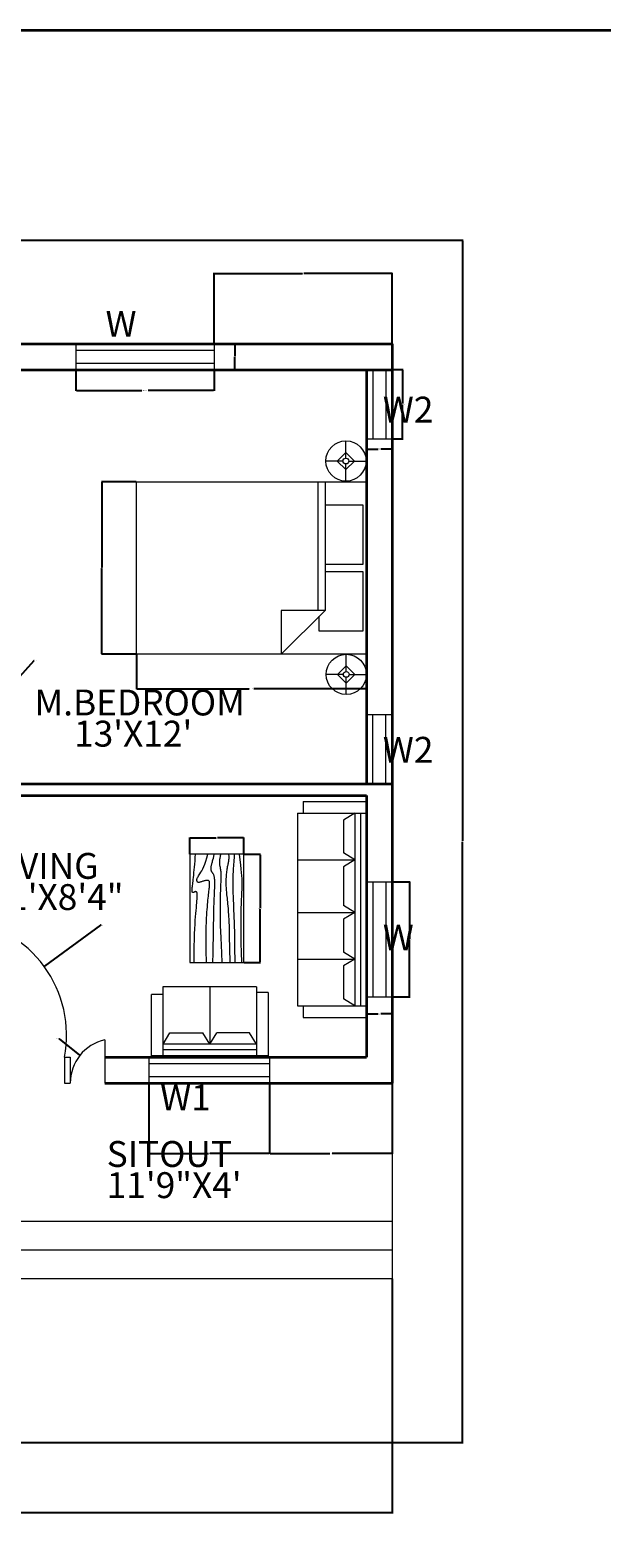
# Model space of a CAD drawing. Units: inches. Extents: x 2473 to 3664, y 1231 to 2079.
# Tile 6 of 8: x 2870 to 3069, y 1555 to 2079. Entities that reach past the tile are written whole.
import ezdxf

# ---------------------------------------------------------------- set-up
doc = ezdxf.new("R2010")
doc.units = ezdxf.units.IN
doc.linetypes.add('ACAD_ISO02W100', pattern=[15, 12, -3])
doc.layers.get('Defpoints').update_dxf_attribs({"linetype": 'ACAD_ISO02W100'})
for name, color, linetype, lineweight in [('A-ANNO-DIMS', 2, 'Continuous', 18), ('A-ANNO-IDEN', 7, 'Continuous', 18), ('A-ANNO-TTLB', 7, 'Continuous', 35), ('A-AREA-IDEN', 7, 'Continuous', 18), ('A-DOOR', 4, 'Continuous', 18), ('A-FLOR-STRS', 7, 'Continuous', 18), ('A-FURN', 8, 'Continuous', 13), ('A-GLAZ', 3, 'Continuous', 18), ('A-WALL', 7, 'Continuous', 35)]:
    doc.layers.add(name, color=color, linetype=linetype, lineweight=lineweight)
doc.styles.get("Standard").update_dxf_attribs({"font": 'arial.ttf'})
doc.dimstyles.get("Standard").update_dxf_attribs({"dimtxt": 0.18, "dimasz": 0.18, "dimexe": 0.18, "dimexo": 0.0625, "dimgap": 0.09, "dimtad": 0, "dimtih": 1, "dimtoh": 1, "dimdec": 4, "dimzin": 0, "dimdsep": 46, "dimtxsty": 'Standard', "dimcen": 0.09, "dimadec": 0, "dimazin": 0, "dimtfac": 1, "dimtdec": 4, "dimtofl": 0, "dimtmove": 0, "dimatfit": 3, "dimfxl": 1, "dimtolj": 1, "dimtzin": 0, "dimarcsym": 0})

# ---------------------------------------------------------------- blocks, each defined once
blk = doc.blocks.new('Bed - Queen')
for p, q in [((0, -80.00003), (0, 0)), ((0, 0), (59.99999, 0)), ((59.99999, 0), (59.99999, -80.00003)), ((7.99999, -1.2), (28.79998, -1.2)), ((7.99999, -14.4), (7.99999, -1.2)), ((28.79998, -1.2), (28.79998, -14.4)), ((31.19999, -1.2), (51.99999, -1.2)), ((31.19999, -14.4), (31.19999, -1.2)), ((51.99999, -1.2), (51.99999, -16.4)), ((0, -14.4), (44.8, -14.4)), ((59.99999, -29.6), (44.8, -14.4)), ((44.8, -14.4), (44.8, -29.6)), ((44.8, -16.8), (0, -16.8)), ((51.99999, -16.4), (46.79936, -16.4)), ((44.8, -29.6), (59.99999, -29.6)), ((59.99999, -80.00003), (0, -80.00003))]:
    blk.add_line(p, q)
blk = doc.blocks.new('Lamp - Table')
for p, q in [((0, 7), (0, 1)), ((-1, 0), (-7, 0)), ((0, 3), (-3, 0)), ((-3, 0), (0, -3)), ((3, 0), (0, 3)), ((0, -3), (3, 0)), ((1, 0), (7, 0)), ((0, -1), (0, -7))]:
    blk.add_line(p, q)
for radius in [7, 1]:
    blk.add_circle((0, 0), radius)
blk = doc.blocks.new('Table - Rectangular Woodgrain 60 x 30 in.')
for p, q in [((0, 0), (0, -30)), ((60, 0), (0, 0)), ((60, -30), (60, 0)), ((0, -30), (60, -30))]:
    blk.add_line(p, q)
for points in [[(0, -2.4), (4.8155, -2.418), (9.0302, -2.4688), (12.709, -2.5477), (15.9167, -2.65), (18.7181, -2.7711), (21.1781, -2.9063), (23.3616, -3.0508), (25.3333, -3.2), (27.1477, -3.3495), (28.8172, -3.4958), (30.3437, -3.636), (31.7291, -3.7667), (32.9756, -3.8849), (34.0849, -3.9875), (35.059, -4.0714), (35.9, -4.1334), (36.6114, -4.1711), (37.2041, -4.1854), (37.6906, -4.1779), (38.0833, -4.15), (38.3948, -4.1034), (38.6375, -4.0396), (38.8239, -3.9602), (38.9666, -3.8667), (39.0764, -3.7608), (39.1573, -3.6448), (39.2116, -3.521), (39.2416, -3.3917), (39.2498, -3.2593), (39.2385, -3.1261), (39.21, -2.9944), (39.1666, -2.8667), (39.111, -2.7447), (39.0468, -2.6281), (38.978, -2.5163), (38.9083, -2.4083), (38.8418, -2.3035), (38.7823, -2.201), (38.7337, -2.1001), (38.7, -2), (38.6844, -1.9003), (38.6875, -1.8021), (38.7094, -1.707), (38.75, -1.6167), (38.8094, -1.5326), (38.8875, -1.4563), (38.9844, -1.3893), (39.1, -1.3333), (39.2351, -1.2896), (39.3937, -1.2583), (39.5804, -1.2396), (39.8, -1.2333), (40.057, -1.2396), (40.3562, -1.2583), (40.7023, -1.2896), (41.1, -1.3333), (41.5547, -1.3895), (42.0755, -1.4573), (42.6721, -1.5361), (43.3542, -1.625), (44.1316, -1.7233), (45.014, -1.8302), (46.0114, -1.9449), (47.1333, -2.0667), (48.3862, -2.1947), (49.7625, -2.3281), (51.2513, -2.4663), (52.8416, -2.6083), (54.5226, -2.7535), (56.2833, -2.9011), (58.1127, -3.0501), (60, -3.2)], [(0, -9.2), (6.5759, -9.0858), (11.9385, -9.0365), (16.2527, -9.0418), (19.6833, -9.0917), (22.3952, -9.1759), (24.5531, -9.2844), (26.322, -9.4069), (27.8666, -9.5333), (29.3241, -9.6553), (30.7203, -9.7719), (32.0532, -9.8837), (33.3208, -9.9917), (34.5213, -10.0965), (35.6526, -10.199), (36.7128, -10.2999), (37.7, -10.4), (38.6129, -10.4996), (39.4531, -10.5969), (40.223, -10.6895), (40.925, -10.775), (41.5613, -10.8512), (42.1344, -10.9156), (42.6465, -10.966), (43.1, -11), (43.4976, -11.0158), (43.8437, -11.0136), (44.143, -10.9942), (44.4, -10.9583), (44.6195, -10.9069), (44.8062, -10.8406), (44.9648, -10.7603), (45.1, -10.6667), (45.2155, -10.5598), (45.3114, -10.4365), (45.3871, -10.2929), (45.4416, -10.125), (45.4743, -9.929), (45.4844, -9.7011), (45.4709, -9.4371), (45.4333, -9.1333), (45.3716, -8.7883), (45.2896, -8.4104), (45.1919, -8.0107), (45.0833, -7.6), (44.9685, -7.1893), (44.8521, -6.7896), (44.7388, -6.4117), (44.6333, -6.0667), (44.54, -5.7628), (44.4614, -5.4979), (44.4001, -5.2675), (44.3583, -5.0667), (44.3384, -4.8909), (44.3427, -4.7354), (44.3736, -4.5956), (44.4333, -4.4667), (44.5236, -4.3453), (44.6427, -4.2333), (44.7884, -4.1339), (44.9583, -4.05), (45.1501, -3.9849), (45.3614, -3.9417), (45.59, -3.9234), (45.8333, -3.9333), (46.0915, -3.9749), (46.3734, -4.0531), (46.6906, -4.1736), (47.0542, -4.3417), (47.4756, -4.5629), (47.9661, -4.8427), (48.5372, -5.1866), (49.2, -5.6), (49.9676, -6.0844), (50.8594, -6.625), (51.8965, -7.2031), (53.1, -7.8), (54.491, -8.3969), (56.0906, -8.975), (57.9199, -9.5156), (60, -10)], [(0, -12.8), (5.1847, -12.9322), (9.6213, -13.0323), (13.3963, -13.1059), (16.5958, -13.1583), (19.3063, -13.1952), (21.614, -13.2219), (23.6054, -13.2439), (25.3666, -13.2667), (26.9728, -13.2947), (28.4531, -13.3281), (29.8256, -13.3663), (31.1083, -13.4083), (32.3191, -13.4535), (33.476, -13.501), (34.597, -13.5501), (35.7, -13.6), (36.7984, -13.6497), (37.8875, -13.6979), (38.9578, -13.743), (40, -13.7833), (41.0047, -13.8174), (41.9625, -13.8438), (42.864, -13.8607), (43.7, -13.8667), (44.4631, -13.8604), (45.1552, -13.8417), (45.7801, -13.8104), (46.3416, -13.7667), (46.8439, -13.7104), (47.2906, -13.6417), (47.6858, -13.5604), (48.0333, -13.4667), (48.3375, -13.3608), (48.6042, -13.2448), (48.8396, -13.121), (49.05, -12.9917), (49.2417, -12.8593), (49.4208, -12.7261), (49.5937, -12.5944), (49.7667, -12.4667), (49.9452, -12.3451), (50.1323, -12.2313), (50.3303, -12.1268), (50.5416, -12.0333), (50.7686, -11.9524), (51.0135, -11.8854), (51.2788, -11.8341), (51.5666, -11.8), (51.8785, -11.7843), (52.2116, -11.7865), (52.562, -11.8059), (52.926, -11.8417), (53.2998, -11.8931), (53.6795, -11.9594), (54.0614, -12.0397), (54.4416, -12.1333), (54.8223, -12.2401), (55.2293, -12.3625), (55.6942, -12.5037), (56.2489, -12.6667), (56.9251, -12.8547), (57.7545, -13.0708), (58.7689, -13.3182), (60, -13.6)], [(0, -18), (5.124, -17.7273), (9.6609, -17.5057), (13.6705, -17.3303), (17.2125, -17.1958), (20.3467, -17.0973), (23.1328, -17.0297), (25.6307, -16.9878), (27.9, -16.9667), (29.9928, -16.9617), (31.9302, -16.9703), (33.7254, -16.9907), (35.3917, -17.0208), (36.9423, -17.0588), (38.3906, -17.1026), (39.7499, -17.1503), (41.0333, -17.2), (42.2519, -17.2496), (43.4073, -17.2969), (44.4986, -17.3395), (45.525, -17.375), (46.4858, -17.4012), (47.3802, -17.4156), (48.2074, -17.416), (48.9667, -17.4), (49.6583, -17.3662), (50.2872, -17.3167), (50.8595, -17.2547), (51.3812, -17.1833), (51.8584, -17.1057), (52.2971, -17.025), (52.7034, -16.9443), (53.0833, -16.8667), (53.443, -16.7951), (53.789, -16.7313), (54.128, -16.6768), (54.4666, -16.6334), (54.8115, -16.6024), (55.1693, -16.5854), (55.5465, -16.5841), (55.95, -16.6), (56.3828, -16.6337), (56.8346, -16.6823), (57.2915, -16.7418), (57.7396, -16.8084), (58.165, -16.878), (58.5539, -16.9469), (58.8924, -17.0111), (59.1666, -17.0667), (59.3679, -17.1107), (59.5078, -17.1438), (59.6032, -17.1675), (59.6708, -17.1833), (59.7275, -17.193), (59.7901, -17.1979), (59.8753, -17.1998), (60, -17.2)], [(0, -22.4), (8.0098, -22.2501), (14.4094, -22.1011), (19.4168, -21.9535), (23.25, -21.8083), (26.1269, -21.6663), (28.2656, -21.5281), (29.884, -21.3947), (31.2, -21.2667), (32.3967, -21.1448), (33.5172, -21.0292), (34.5697, -20.9198), (35.5625, -20.8167), (36.5037, -20.7198), (37.4015, -20.6292), (38.2642, -20.5448), (39.1, -20.4667), (39.9164, -20.3951), (40.7187, -20.3313), (41.5117, -20.2768), (42.3, -20.2333), (43.0883, -20.2024), (43.8812, -20.1854), (44.6836, -20.1841), (45.5, -20.2), (46.3328, -20.234), (47.1747, -20.2844), (48.0163, -20.3488), (48.8479, -20.425), (49.66, -20.5106), (50.4429, -20.6031), (51.1872, -20.7004), (51.8833, -20.8), (52.5246, -20.8999), (53.1166, -20.9995), (53.6681, -21.0983), (54.1875, -21.1958), (54.6834, -21.2919), (55.1646, -21.3859), (55.6394, -21.4777), (56.1167, -21.5667), (56.6028, -21.6515), (57.0961, -21.7266), (57.5929, -21.7852), (58.0896, -21.8208), (58.5823, -21.8268), (59.0674, -21.7964), (59.5412, -21.723), (60, -21.6)], [(0, -25.2), (8.6355, -25.0504), (15.7026, -24.9031), (21.4049, -24.7606), (25.9458, -24.625), (29.529, -24.4988), (32.3578, -24.3844), (34.6359, -24.284), (36.5667, -24.2), (38.3213, -24.1341), (39.9417, -24.0854), (41.437, -24.0523), (42.8167, -24.0333), (44.0901, -24.0268), (45.2667, -24.0313), (46.3557, -24.0451), (47.3667, -24.0667), (48.309, -24.0947), (49.1928, -24.1287), (50.0284, -24.168), (50.826, -24.2125), (51.5959, -24.2617), (52.3483, -24.3151), (53.0935, -24.3725), (53.8417, -24.4334), (54.6009, -24.497), (55.3699, -24.561), (56.1454, -24.6226), (56.9239, -24.6792), (57.7021, -24.7279), (58.4764, -24.7662), (59.2435, -24.7911), (60, -24.8)], [(0, -28.8), (5.6867, -28.6681), (10.45, -28.5698), (14.407, -28.5012), (17.675, -28.4584), (20.3711, -28.4374), (22.6125, -28.4344), (24.5164, -28.4455), (26.2, -28.4667), (27.762, -28.4947), (29.2276, -28.5281), (30.6033, -28.5663), (31.8958, -28.6084), (33.1118, -28.6535), (34.2578, -28.7011), (35.3405, -28.7501), (36.3666, -28.8), (37.3443, -28.8497), (38.288, -28.8974), (39.2137, -28.9412), (40.1375, -28.9792), (41.0753, -29.0093), (42.0432, -29.0297), (43.0572, -29.0384), (44.1333, -29.0333), (45.2936, -29.0114), (46.5843, -28.9641), (48.0579, -28.8816), (49.7666, -28.7542), (51.7629, -28.5721), (54.0989, -28.3255), (56.8272, -28.0048), (60, -27.6)]]:
    blk.add_lwpolyline(points)
blk = doc.blocks.new('GLAZ-PLAN-48')
for p, q in [((0, 9), (0, 0)), ((0, 6.75), (48, 6.75)), ((48, 9), (48, 0)), ((0, 2.25), (48, 2.25))]:
    blk.add_line(p, q)
blk = doc.blocks.new('GLAZ-PLAN-40')
for p, q in [((0, 40), (9, 40)), ((2.25, 40), (2.25, 0)), ((6.75, 40), (6.75, 0)), ((0, 0), (9, 0))]:
    blk.add_line(p, q)
blk = doc.blocks.new('GLAZ-PLAN-24-END')
for p, q in [((2.25, 24), (2.25, 0)), ((6.75, 24), (6.75, 0)), ((0, 0), (9, 0))]:
    blk.add_line(p, q)
blk = doc.blocks.new('STEPS-SITOUT-PLAN')
for p, q in [((151, 68), (151, 0)), ((0, 20), (151, 20)), ((0, 10), (151, 10)), ((0, 0), (151, 0))]:
    blk.add_line(p, q)
blk = doc.blocks.new('*D21')
at = {"layer": 'A-ANNO-DIMS', "color": 0, "lineweight": -2, "transparency": 16777216}
for p, q in [((2885.66, 1960.99), (2885.66, 1953.68)), ((2933.66, 1960.99), (2933.66, 1953.68)), ((2885.84, 1953.86), (2908.54, 1953.86)), ((2933.48, 1953.86), (2910.78, 1953.86))]:
    blk.add_line(p, q, dxfattribs=at)
at = {"layer": 'A-ANNO-DIMS', "color": 0, "transparency": 16777216}
for points in [[(2885.84, 1953.89), (2885.84, 1953.83), (2885.66, 1953.86)], [(2933.48, 1953.89), (2933.48, 1953.83), (2933.66, 1953.86)]]:
    blk.add_solid(points, dxfattribs=at)
at = {"layer": 'Defpoints', "color": 0, "transparency": 16777216}
for p in [(2885.66, 1961.06), (2933.66, 1961.06), (2933.66, 1953.86)]:
    blk.add_point(p, dxfattribs=at)
at = {"layer": 'A-ANNO-DIMS', "color": 0, "transparency": 16777216, "insert": (2909.66, 1953.86), "char_height": 0.18, "attachment_point": 5}
blk.add_mtext('\\A1;WINDOW 48 TYP.', dxfattribs=at)
blk = doc.blocks.new('*D22')
at = {"layer": 'A-ANNO-DIMS', "color": 0, "lineweight": -2, "transparency": 16777216}
for p, q in [((2933.72, 1970.06), (2941.04, 1970.06)), ((2940.86, 1969.88), (2940.86, 1965.74)), ((2933.72, 1961.06), (2941.04, 1961.06)), ((2940.86, 1961.24), (2940.86, 1965.37))]:
    blk.add_line(p, q, dxfattribs=at)
at = {"layer": 'A-ANNO-DIMS', "color": 0, "transparency": 16777216}
for points in [[(2940.83, 1969.88), (2940.89, 1969.88), (2940.86, 1970.06)], [(2940.83, 1961.24), (2940.89, 1961.24), (2940.86, 1961.06)]]:
    blk.add_solid(points, dxfattribs=at)
at = {"layer": 'Defpoints', "color": 0, "transparency": 16777216}
for p in [(2933.66, 1970.06), (2940.86, 1970.06), (2933.66, 1961.06)]:
    blk.add_point(p, dxfattribs=at)
at = {"layer": 'A-ANNO-DIMS', "color": 0, "transparency": 16777216, "insert": (2940.86, 1965.56), "char_height": 0.18, "attachment_point": 5}
blk.add_mtext('\\A1;9 TYP.', dxfattribs=at)
blk = doc.blocks.new('*D25')
at = {"layer": 'A-ANNO-DIMS', "color": 0, "lineweight": -2, "transparency": 16777216}
for p, q in [((2906.66, 1862.06), (2906.66, 1849.94)), ((2986.66, 1862.06), (2986.66, 1849.94)), ((2906.84, 1850.12), (2945.84, 1850.12)), ((2986.48, 1850.12), (2947.48, 1850.12))]:
    blk.add_line(p, q, dxfattribs=at)
at = {"layer": 'A-ANNO-DIMS', "color": 0, "transparency": 16777216}
for points in [[(2906.84, 1850.15), (2906.84, 1850.09), (2906.66, 1850.12)], [(2986.48, 1850.15), (2986.48, 1850.09), (2986.66, 1850.12)]]:
    blk.add_solid(points, dxfattribs=at)
at = {"layer": 'Defpoints', "color": 0, "transparency": 16777216}
for p in [(2906.66, 1862.12), (2986.66, 1862.12), (2986.66, 1850.12)]:
    blk.add_point(p, dxfattribs=at)
at = {"layer": 'A-ANNO-DIMS', "color": 0, "transparency": 16777216, "insert": (2946.66, 1850.12), "char_height": 0.18, "attachment_point": 5}
blk.add_mtext('\\A1;BED 80 TYP.', dxfattribs=at)
blk = doc.blocks.new('*D26')
at = {"layer": 'A-ANNO-DIMS', "color": 0, "lineweight": -2, "transparency": 16777216}
for p, q in [((2906.6, 1922.12), (2894.48, 1922.12)), ((2894.66, 1921.94), (2894.66, 1892.3)), ((2894.66, 1862.3), (2894.66, 1891.94)), ((2906.6, 1862.12), (2894.48, 1862.12))]:
    blk.add_line(p, q, dxfattribs=at)
at = {"layer": 'A-ANNO-DIMS', "color": 0, "transparency": 16777216}
for points in [[(2894.63, 1921.94), (2894.69, 1921.94), (2894.66, 1922.12)], [(2894.63, 1862.3), (2894.69, 1862.3), (2894.66, 1862.12)]]:
    blk.add_solid(points, dxfattribs=at)
at = {"layer": 'Defpoints', "color": 0, "transparency": 16777216}
for p in [(2906.66, 1922.12), (2894.66, 1862.12), (2906.66, 1862.12)]:
    blk.add_point(p, dxfattribs=at)
at = {"layer": 'A-ANNO-DIMS', "color": 0, "transparency": 16777216, "insert": (2894.66, 1892.12), "char_height": 0.18, "attachment_point": 5}
blk.add_mtext('\\A1;60 TYP.', dxfattribs=at)
blk = doc.blocks.new('*D27')
at = {"layer": 'A-ANNO-DIMS', "color": 0, "lineweight": -2, "transparency": 16777216}
for p, q in [((2995.72, 1783.06), (3001.84, 1783.06)), ((3001.66, 1782.88), (3001.66, 1763.24)), ((3001.66, 1743.24), (3001.66, 1762.87)), ((2995.72, 1743.06), (3001.84, 1743.06))]:
    blk.add_line(p, q, dxfattribs=at)
at = {"layer": 'A-ANNO-DIMS', "color": 0, "transparency": 16777216}
for points in [[(3001.63, 1782.88), (3001.69, 1782.88), (3001.66, 1783.06)], [(3001.63, 1743.24), (3001.69, 1743.24), (3001.66, 1743.06)]]:
    blk.add_solid(points, dxfattribs=at)
at = {"layer": 'Defpoints', "color": 0, "transparency": 16777216}
for p in [(2995.66, 1783.06), (3001.66, 1783.06), (2995.66, 1743.06)]:
    blk.add_point(p, dxfattribs=at)
at = {"layer": 'A-ANNO-DIMS', "color": 0, "transparency": 16777216, "insert": (3001.66, 1763.06), "char_height": 0.18, "attachment_point": 5}
blk.add_mtext('\\A1;WINDOW 40 TYP.', dxfattribs=at)
blk = doc.blocks.new('*D28')
at = {"layer": 'A-ANNO-DIMS', "color": 0, "lineweight": -2, "transparency": 16777216}
for p, q in [((2986.66, 1742.99), (2986.66, 1736.88)), ((2995.66, 1742.99), (2995.66, 1736.88)), ((2986.84, 1737.06), (2990.7, 1737.06)), ((2995.48, 1737.06), (2991.62, 1737.06))]:
    blk.add_line(p, q, dxfattribs=at)
at = {"layer": 'A-ANNO-DIMS', "color": 0, "transparency": 16777216}
for points in [[(2986.84, 1737.09), (2986.84, 1737.03), (2986.66, 1737.06)], [(2995.48, 1737.09), (2995.48, 1737.03), (2995.66, 1737.06)]]:
    blk.add_solid(points, dxfattribs=at)
at = {"layer": 'Defpoints', "color": 0, "transparency": 16777216}
for p in [(2986.66, 1743.06), (2995.66, 1743.06), (2995.66, 1737.06)]:
    blk.add_point(p, dxfattribs=at)
at = {"layer": 'A-ANNO-DIMS', "color": 0, "transparency": 16777216, "insert": (2991.16, 1737.06), "char_height": 0.18, "attachment_point": 5}
blk.add_mtext('\\A1;9 TYP.', dxfattribs=at)
blk = doc.blocks.new('*D33')
at = {"layer": 'A-ANNO-DIMS', "color": 0, "lineweight": -2, "transparency": 16777216}
for p, q in [((2995.72, 1961.06), (2999.44, 1961.06)), ((2999.26, 1960.88), (2999.26, 1949.24)), ((2999.26, 1937.24), (2999.26, 1948.87)), ((2995.72, 1937.06), (2999.44, 1937.06))]:
    blk.add_line(p, q, dxfattribs=at)
at = {"layer": 'A-ANNO-DIMS', "color": 0, "transparency": 16777216}
for points in [[(2999.23, 1960.88), (2999.29, 1960.88), (2999.26, 1961.06)], [(2999.23, 1937.24), (2999.29, 1937.24), (2999.26, 1937.06)]]:
    blk.add_solid(points, dxfattribs=at)
at = {"layer": 'Defpoints', "color": 0, "transparency": 16777216}
for p in [(2995.66, 1961.06), (2999.26, 1961.06), (2995.66, 1937.06)]:
    blk.add_point(p, dxfattribs=at)
at = {"layer": 'A-ANNO-DIMS', "color": 0, "transparency": 16777216, "insert": (2999.26, 1949.06), "char_height": 0.18, "attachment_point": 5}
blk.add_mtext('\\A1;WINDOW 24 TYP.', dxfattribs=at)
blk = doc.blocks.new('*D34')
at = {"layer": 'A-ANNO-DIMS', "color": 0, "lineweight": -2, "transparency": 16777216}
for p, q in [((2986.66, 1936.99), (2986.66, 1933.28)), ((2995.66, 1936.99), (2995.66, 1933.28)), ((2986.84, 1933.46), (2990.7, 1933.46)), ((2995.48, 1933.46), (2991.62, 1933.46))]:
    blk.add_line(p, q, dxfattribs=at)
at = {"layer": 'A-ANNO-DIMS', "color": 0, "transparency": 16777216}
for points in [[(2986.84, 1933.49), (2986.84, 1933.43), (2986.66, 1933.46)], [(2995.48, 1933.49), (2995.48, 1933.43), (2995.66, 1933.46)]]:
    blk.add_solid(points, dxfattribs=at)
at = {"layer": 'Defpoints', "color": 0, "transparency": 16777216}
for p in [(2986.66, 1937.06), (2995.66, 1937.06), (2995.66, 1933.46)]:
    blk.add_point(p, dxfattribs=at)
at = {"layer": 'A-ANNO-DIMS', "color": 0, "transparency": 16777216, "insert": (2991.16, 1933.46), "char_height": 0.18, "attachment_point": 5}
blk.add_mtext('\\A1;9 TYP.', dxfattribs=at)
blk = doc.blocks.new('*D47')
at = {"layer": 'A-ANNO-DIMS', "color": 0, "lineweight": -2, "transparency": 16777216}
for p, q in [((2944.12, 1792.62), (2949.88, 1792.62)), ((2949.7, 1792.44), (2949.7, 1773.98)), ((2949.7, 1755.15), (2949.7, 1773.61)), ((2944.12, 1754.97), (2949.88, 1754.97))]:
    blk.add_line(p, q, dxfattribs=at)
at = {"layer": 'A-ANNO-DIMS', "color": 0, "transparency": 16777216}
for points in [[(2949.67, 1792.44), (2949.73, 1792.44), (2949.7, 1792.62)], [(2949.67, 1755.15), (2949.73, 1755.15), (2949.7, 1754.97)]]:
    blk.add_solid(points, dxfattribs=at)
at = {"layer": 'Defpoints', "color": 0, "transparency": 16777216}
for p in [(2944.06, 1792.62), (2949.7, 1792.62), (2944.06, 1754.97)]:
    blk.add_point(p, dxfattribs=at)
at = {"layer": 'A-ANNO-DIMS', "color": 0, "transparency": 16777216, "insert": (2949.7, 1773.8), "char_height": 0.18, "attachment_point": 5}
blk.add_mtext('\\A1;TABLE 38', dxfattribs=at)
blk = doc.blocks.new('*D48')
at = {"layer": 'A-ANNO-DIMS', "color": 0, "lineweight": -2, "transparency": 16777216}
for p, q in [((2925.23, 1792.68), (2925.23, 1798.45)), ((2925.41, 1798.27), (2934.43, 1798.27)), ((2943.88, 1798.27), (2934.86, 1798.27)), ((2944.06, 1792.68), (2944.06, 1798.45))]:
    blk.add_line(p, q, dxfattribs=at)
at = {"layer": 'A-ANNO-DIMS', "color": 0, "transparency": 16777216}
for points in [[(2925.41, 1798.3), (2925.41, 1798.24), (2925.23, 1798.27)], [(2943.88, 1798.3), (2943.88, 1798.24), (2944.06, 1798.27)]]:
    blk.add_solid(points, dxfattribs=at)
at = {"layer": 'Defpoints', "color": 0, "transparency": 16777216}
for p in [(2925.23, 1798.27), (2925.23, 1792.62), (2944.06, 1792.62)]:
    blk.add_point(p, dxfattribs=at)
at = {"layer": 'A-ANNO-DIMS', "color": 0, "transparency": 16777216, "insert": (2934.64, 1798.27), "char_height": 0.18, "attachment_point": 5}
blk.add_mtext('\\A1;19', dxfattribs=at)
blk = doc.blocks.new('*D49')
at = {"layer": 'A-ANNO-DIMS', "color": 0, "lineweight": -2, "transparency": 16777216}
for p, q in [((2995.66, 1644.99), (2995.66, 1563.43)), ((2617.66, 1587.99), (2617.66, 1563.43)), ((2617.84, 1563.61), (2806.37, 1563.61)), ((2995.48, 1563.61), (2806.95, 1563.61))]:
    blk.add_line(p, q, dxfattribs=at)
at = {"layer": 'A-ANNO-DIMS', "color": 0, "transparency": 16777216}
for points in [[(2617.84, 1563.64), (2617.84, 1563.58), (2617.66, 1563.61)], [(2995.48, 1563.64), (2995.48, 1563.58), (2995.66, 1563.61)]]:
    blk.add_solid(points, dxfattribs=at)
at = {"layer": 'Defpoints', "color": 0, "transparency": 16777216}
for p in [(2995.66, 1645.06), (2617.66, 1588.06), (2995.66, 1563.61)]:
    blk.add_point(p, dxfattribs=at)
at = {"layer": 'A-ANNO-DIMS', "color": 0, "transparency": 16777216, "insert": (2806.66, 1563.61), "char_height": 0.18, "attachment_point": 5}
blk.add_mtext('\\A1;378', dxfattribs=at)
blk = doc.blocks.new('*D50')
at = {"layer": 'A-ANNO-DIMS', "color": 0, "lineweight": -2, "transparency": 16777216}
for p, q in [((2746.72, 2006.06), (3020.29, 2006.06)), ((3020.11, 2005.88), (3020.11, 1797.24)), ((3020.11, 1588.24), (3020.11, 1796.87)), ((2844.72, 1588.06), (3020.29, 1588.06))]:
    blk.add_line(p, q, dxfattribs=at)
at = {"layer": 'A-ANNO-DIMS', "color": 0, "transparency": 16777216}
for points in [[(3020.08, 2005.88), (3020.14, 2005.88), (3020.11, 2006.06)], [(3020.08, 1588.24), (3020.14, 1588.24), (3020.11, 1588.06)]]:
    blk.add_solid(points, dxfattribs=at)
at = {"layer": 'Defpoints', "color": 0, "transparency": 16777216}
for p in [(2746.66, 2006.06), (3020.11, 2006.06), (2844.66, 1588.06)]:
    blk.add_point(p, dxfattribs=at)
at = {"layer": 'A-ANNO-DIMS', "color": 0, "transparency": 16777216, "insert": (3020.11, 1797.06), "char_height": 0.18, "attachment_point": 5}
blk.add_mtext('\\A1;418', dxfattribs=at)
blk = doc.blocks.new('*D55')
at = {"layer": 'A-ANNO-DIMS', "color": 0, "lineweight": -2, "transparency": 16777216}
for p, q in [((2933.66, 1970.12), (2933.66, 1994.69)), ((2933.84, 1994.51), (2964.44, 1994.51)), ((2995.48, 1994.51), (2964.88, 1994.51)), ((2995.66, 1970.12), (2995.66, 1994.69))]:
    blk.add_line(p, q, dxfattribs=at)
at = {"layer": 'A-ANNO-DIMS', "color": 0, "transparency": 16777216}
for points in [[(2933.84, 1994.54), (2933.84, 1994.48), (2933.66, 1994.51)], [(2995.48, 1994.54), (2995.48, 1994.48), (2995.66, 1994.51)]]:
    blk.add_solid(points, dxfattribs=at)
at = {"layer": 'Defpoints', "color": 0, "transparency": 16777216}
for p in [(2995.66, 1994.51), (2933.66, 1970.06), (2995.66, 1970.06)]:
    blk.add_point(p, dxfattribs=at)
at = {"layer": 'A-ANNO-DIMS', "color": 0, "transparency": 16777216, "insert": (2964.66, 1994.51), "char_height": 0.18, "attachment_point": 5}
blk.add_mtext('\\A1;62', dxfattribs=at)
blk = doc.blocks.new('*D61')
at = {"layer": 'A-ANNO-DIMS', "color": 0, "lineweight": -2, "transparency": 16777216}
for p, q in [((2911.01, 1712.99), (2911.01, 1688.43)), ((2953.01, 1712.99), (2953.01, 1688.43)), ((2911.19, 1688.61), (2931.79, 1688.61)), ((2952.83, 1688.61), (2932.23, 1688.61))]:
    blk.add_line(p, q, dxfattribs=at)
at = {"layer": 'A-ANNO-DIMS', "color": 0, "transparency": 16777216}
for points in [[(2911.19, 1688.64), (2911.19, 1688.58), (2911.01, 1688.61)], [(2952.83, 1688.64), (2952.83, 1688.58), (2953.01, 1688.61)]]:
    blk.add_solid(points, dxfattribs=at)
at = {"layer": 'Defpoints', "color": 0, "transparency": 16777216}
for p in [(2911.01, 1713.06), (2953.01, 1713.06), (2911.01, 1688.61)]:
    blk.add_point(p, dxfattribs=at)
at = {"layer": 'A-ANNO-DIMS', "color": 0, "transparency": 16777216, "insert": (2932.01, 1688.61), "char_height": 0.18, "attachment_point": 5}
blk.add_mtext('\\A1;42', dxfattribs=at)
blk = doc.blocks.new('*D62')
at = {"layer": 'A-ANNO-DIMS', "color": 0, "lineweight": -2, "transparency": 16777216}
for p, q in [((2953.01, 1712.99), (2953.01, 1688.43)), ((2995.66, 1712.99), (2995.66, 1688.43)), ((2953.19, 1688.61), (2973.94, 1688.61)), ((2995.48, 1688.61), (2974.73, 1688.61))]:
    blk.add_line(p, q, dxfattribs=at)
at = {"layer": 'A-ANNO-DIMS', "color": 0, "transparency": 16777216}
for points in [[(2953.19, 1688.64), (2953.19, 1688.58), (2953.01, 1688.61)], [(2995.48, 1688.64), (2995.48, 1688.58), (2995.66, 1688.61)]]:
    blk.add_solid(points, dxfattribs=at)
at = {"layer": 'Defpoints', "color": 0, "transparency": 16777216}
for p in [(2953.01, 1713.06), (2995.66, 1713.06), (2953.01, 1688.61)]:
    blk.add_point(p, dxfattribs=at)
at = {"layer": 'A-ANNO-DIMS', "color": 0, "transparency": 16777216, "insert": (2974.34, 1688.61), "char_height": 0.18, "attachment_point": 5}
blk.add_mtext('\\A1;42.65', dxfattribs=at)
blk = doc.blocks.new('*D105')
at = {"layer": 'A-ANNO-DIMS', "color": 0, "lineweight": -2, "transparency": 16777216}
for p, q in [((2894.18, 1767.94), (2874.73, 1753.71)), ((2894.36, 1767.94), (2894.18, 1767.94)), ((2841.83, 1729.71), (2842.01, 1729.71)), ((2841.92, 1729.62), (2841.92, 1729.8))]:
    blk.add_line(p, q, dxfattribs=at)
at = {"layer": 'A-ANNO-DIMS', "color": 0, "transparency": 16777216}
blk.add_solid([(2874.71, 1753.73), (2874.75, 1753.68), (2874.58, 1753.6)], dxfattribs=at)
at = {"layer": 'Defpoints', "color": 0, "transparency": 16777216}
for p in [(2874.58, 1753.6), (2841.92, 1729.71)]:
    blk.add_point(p, dxfattribs=at)
at = {"layer": 'A-ANNO-DIMS', "color": 0, "transparency": 16777216, "insert": (2894.84, 1767.94), "char_height": 0.18, "attachment_point": 5}
blk.add_mtext('\\A1;R40.47', dxfattribs=at)
blk = doc.blocks.new('*D108')
at = {"layer": 'A-ANNO-DIMS', "color": 0, "lineweight": -2, "transparency": 16777216}
for p, q in [((2870.98, 1859.89), (2857.23, 1844.52)), ((2871.16, 1859.89), (2870.98, 1859.89)), ((2833.9, 1818.54), (2834.08, 1818.54)), ((2833.99, 1818.45), (2833.99, 1818.63))]:
    blk.add_line(p, q, dxfattribs=at)
at = {"layer": 'A-ANNO-DIMS', "color": 0, "transparency": 16777216}
blk.add_solid([(2857.21, 1844.54), (2857.25, 1844.5), (2857.11, 1844.38)], dxfattribs=at)
at = {"layer": 'Defpoints', "color": 0, "transparency": 16777216}
for p in [(2857.11, 1844.38), (2833.99, 1818.54)]:
    blk.add_point(p, dxfattribs=at)
at = {"layer": 'A-ANNO-DIMS', "color": 0, "transparency": 16777216, "insert": (2871.64, 1859.89), "char_height": 0.18, "attachment_point": 5}
blk.add_mtext('\\A1;R34.68', dxfattribs=at)
blk = doc.blocks.new('*D111')
at = {"layer": 'A-ANNO-DIMS', "color": 0, "lineweight": -2, "transparency": 16777216}
for p, q in [((2879.65, 1728.42), (2879.83, 1728.42)), ((2879.83, 1728.42), (2886.89, 1722.77)), ((2898.95, 1713.06), (2899.13, 1713.06)), ((2899.04, 1712.97), (2899.04, 1713.15))]:
    blk.add_line(p, q, dxfattribs=at)
at = {"layer": 'A-ANNO-DIMS', "color": 0, "transparency": 16777216}
blk.add_solid([(2886.91, 1722.8), (2886.87, 1722.75), (2887.03, 1722.66)], dxfattribs=at)
at = {"layer": 'Defpoints', "color": 0, "transparency": 16777216}
for p in [(2887.03, 1722.66), (2899.04, 1713.06)]:
    blk.add_point(p, dxfattribs=at)
at = {"layer": 'A-ANNO-DIMS', "color": 0, "transparency": 16777216, "insert": (2879.1, 1728.42), "char_height": 0.18, "attachment_point": 5}
blk.add_mtext('\\A1;R15.375', dxfattribs=at)

msp = doc.modelspace()

# ---------------------------------------------------------------- linework, layer by layer
at = {"layer": 'A-ANNO-TTLB'}
msp.add_lwpolyline([(2473.2801, 2079.0861), (3663.7983, 2079.0861), (3663.7983, 1231.3065), (2473.2801, 1231.3065)], close=True, dxfattribs=at)
at = {"layer": 'A-DOOR'}
for p, q in [((2881.6604, 1737.0561), (2881.7176, 1737.0561)), ((2895.6604, 1728.0561), (2895.6604, 1713.0561)), ((2881.6604, 1722.0561), (2881.6604, 1713.0561)), ((2881.6604, 1722.0561), (2883.6604, 1722.0561)), ((2883.6604, 1722.0561), (2883.6604, 1713.0561)), ((2881.6604, 1713.0561), (2883.6604, 1713.0561))]:
    msp.add_line(p, q, dxfattribs=at)
for centre, radius, start, end in [((2841.9202, 1729.7076), 40.4701, 349.101732, 83.273573), ((2899.0354, 1713.0561), 15.375, 102.680383, 180)]:
    msp.add_arc(centre, radius, start, end, dxfattribs=at)
at = {"layer": 'A-FURN'}
for p, q in [((2964.6604, 1810.9003), (2964.6604, 1806.9003)), ((2964.6604, 1810.9003), (2986.6604, 1810.9003)), ((2962.6604, 1806.9003), (2986.6604, 1806.9003)), ((2962.6604, 1806.9003), (2962.6604, 1739.9003)), ((2982.6604, 1806.9003), (2978.6604, 1804.4972)), ((2978.6604, 1804.4972), (2978.6604, 1793.0534)), ((2982.6604, 1806.9003), (2982.6604, 1739.9003)), ((2984.6604, 1806.9003), (2984.6604, 1739.9003)), ((2982.6604, 1790.6503), (2978.6604, 1793.0534)), ((2962.6604, 1790.6503), (2982.6604, 1790.6503)), ((2982.6604, 1790.6503), (2978.6604, 1788.2472)), ((2978.6604, 1788.2472), (2978.6604, 1774.8034)), ((2962.6604, 1772.4003), (2982.6604, 1772.4003)), ((2982.6604, 1772.4003), (2978.6604, 1774.8034)), ((2982.6604, 1772.4003), (2978.6604, 1769.9972)), ((2978.6604, 1769.9972), (2978.6604, 1758.5534)), ((2978.6604, 1769.9972), (2978.6604, 1758.5534)), ((2962.6604, 1756.1503), (2982.6604, 1756.1503)), ((2982.6604, 1756.1503), (2978.6604, 1758.5534)), ((2982.6604, 1756.1503), (2978.6604, 1753.7472)), ((2978.6604, 1753.7472), (2978.6604, 1742.3034)), ((2978.6604, 1753.7472), (2978.6604, 1742.3034)), ((2948.4417, 1746.5613), (2915.8903, 1746.5613)), ((2915.8903, 1746.5613), (2915.8903, 1722.5613)), ((2932.1917, 1746.5613), (2932.1917, 1726.5613)), ((2932.1917, 1746.5613), (2932.1917, 1726.5613)), ((2948.4417, 1746.5613), (2948.4417, 1722.5613)), ((2915.8903, 1743.7811), (2911.8903, 1743.7811)), ((2911.8903, 1722.5613), (2911.8903, 1743.7811)), ((2952.4417, 1744.5613), (2948.4417, 1744.5613)), ((2952.4417, 1744.5613), (2952.4417, 1722.5613)), ((2982.6604, 1739.9003), (2978.6604, 1742.3034)), ((2962.6604, 1739.9003), (2986.6604, 1739.9003)), ((2964.6604, 1739.9003), (2964.6604, 1735.9003)), ((2964.6604, 1735.9003), (2986.6604, 1735.9003)), ((2915.9417, 1726.5613), (2918.3448, 1730.5613)), ((2918.3448, 1730.5613), (2929.7886, 1730.5613)), ((2932.1917, 1726.5613), (2929.7886, 1730.5613)), ((2932.1917, 1726.5613), (2934.5948, 1730.5613)), ((2946.0386, 1730.5613), (2934.5948, 1730.5613)), ((2948.4417, 1726.5613), (2946.0386, 1730.5613)), ((2948.4417, 1726.5613), (2915.8903, 1726.5613)), ((2948.4417, 1724.5613), (2915.8903, 1724.5613)), ((2952.4417, 1722.5613), (2911.8903, 1722.5613))]:
    msp.add_line(p, q, dxfattribs=at)
at = {"layer": 'A-GLAZ'}
for p, q in [((2988.9104, 1783.0561), (2988.9104, 1743.0561)), ((2993.4104, 1783.0561), (2993.4104, 1743.0561)), ((2911.0131, 1722.0561), (2911.0131, 1713.0561)), ((2911.0131, 1719.8061), (2953.0131, 1719.8061)), ((2953.0131, 1722.0561), (2953.0131, 1713.0561)), ((2911.0131, 1715.3061), (2953.0131, 1715.3061))]:
    msp.add_line(p, q, dxfattribs=at)
at = {"layer": 'A-WALL'}
for p, q in [((2728.6604, 1970.0561), (2995.6604, 1970.0561)), ((2995.6604, 1970.0561), (2995.6604, 1713.0561)), ((2830.6604, 1961.0561), (2995.6604, 1961.0561)), ((2986.6604, 1961.0561), (2986.6604, 1817.0561)), ((2830.6604, 1817.0561), (2995.6604, 1817.0561)), ((2826.6604, 1813.0561), (2986.6604, 1813.0561)), ((2986.6604, 1813.0561), (2986.6604, 1722.0561)), ((2895.6604, 1722.0561), (2986.6604, 1722.0561)), ((2895.6604, 1713.0561), (2995.6604, 1713.0561))]:
    msp.add_line(p, q, dxfattribs=at)

# ---------------------------------------------------------------- block references
at = {"layer": 'A-FLOR-STRS'}
msp.add_blockref('STEPS-SITOUT-PLAN', (2844.66, 1645.056), dxfattribs=at)
at = {"layer": 'A-FURN'}
for name, p, rotation in [('Lamp - Table', (2979.5445, 1929.2959), 180), ('Bed - Queen', (2986.6604, 1922.1196), 270), ('Lamp - Table', (2979.6604, 1855.11), 180)]:
    msp.add_blockref(name, p, dxfattribs=dict(at, rotation=rotation))
at = {"layer": 'A-FURN', "xscale": 0.6274050888137993, "yscale": 0.6274050888137993, "zscale": 0.6274050888137993, "rotation": 90}
msp.add_blockref('Table - Rectangular Woodgrain 60 x 30 in.', (2925.2335, 1754.9745), dxfattribs=at)
at = {"layer": 'A-GLAZ'}
for name, p in [('GLAZ-PLAN-48', (2885.66, 1961.056)), ('GLAZ-PLAN-24-END', (2986.66, 1937.056)), ('GLAZ-PLAN-40', (2986.66, 1743.056))]:
    msp.add_blockref(name, p, dxfattribs=at)
at = {"layer": 'A-GLAZ', "rotation": 180}
msp.add_blockref('GLAZ-PLAN-24-END', (2995.6608, 1841.0562), dxfattribs=at)

# ---------------------------------------------------------------- texts
at = {"layer": 'A-ANNO-IDEN'}
for s, p in [('           W', (2865.6814, 1972.4987)), ('           W2', (2962.1134, 1942.6621)), ('           W2', (2962.1134, 1824.3968)), ('           W', (2962.1134, 1759.1358)), ('           W1', (2884.6847, 1703.5386))]:
    msp.add_text(s, height=9, dxfattribs=at).set_placement(p)
at = {"layer": 'A-AREA-IDEN'}
for s, p in [('M.BEDROOM', (2871.2406, 1840.8559)), ("     13'X12'", (2871.2406, 1830.0177)), (' LIVING', (2852.4886, 1784.047)), (' 11\'X8\'4"', (2852.4886, 1773.2089)), (' SITOUT', (2893.5817, 1683.8933)), (' 11\'9"X4\'', (2893.5817, 1673.0551))]:
    msp.add_text(s, height=9, dxfattribs=at).set_placement(p)

# ---------------------------------------------------------------- dimensions: what is measured, and where the dimension line sits
at = {"layer": 'A-ANNO-DIMS'}
for base, p1, p2, angle, override, picture, middle in [((3020.1104, 2006.0561), (2844.6604, 1588.0561), (2746.6604, 2006.0561), 90, {"dimdec": 0, "dimlfac": 1, "dimrnd": 0, "dimzin": 0, "dimdsep": 46, "dimlunit": 2}, '*D50', (3020.1104, 1797.0561)), ((2925.2335, 1798.2654), (2944.0557, 1792.6188), (2925.2335, 1792.6188), 180, {"dimdec": 0, "dimlfac": 1, "dimrnd": 0, "dimzin": 0, "dimdsep": 46, "dimlunit": 2}, '*D48', (2934.6446, 1798.2654)), ((2911.0131, 1688.6061), (2953.0131, 1713.0561), (2911.0131, 1713.0561), 180, {"dimdec": 0, "dimlfac": 1, "dimrnd": 0, "dimzin": 0, "dimdsep": 46, "dimlunit": 2}, '*D61', (2932.0131, 1688.6061)), ((2953.0131, 1688.6061), (2995.6604, 1713.0561), (2953.0131, 1713.0561), 180, {"dimdec": 2, "dimlfac": 1, "dimrnd": 0, "dimzin": 0, "dimdsep": 46, "dimlunit": 2}, '*D62', (2974.3368, 1688.6061))]:
    dim = msp.add_linear_dim(base=base, p1=p1, p2=p2, angle=angle, dimstyle='Standard', override=override, dxfattribs=at)
    dim.commit()
    dim.dimension.update_dxf_attribs({"geometry": picture, "text_midpoint": middle})
for base, p1, p2, picture, middle in [((2995.6604, 1994.5061), (2933.6604, 1970.0561), (2995.6604, 1970.0561), '*D55', (2964.6604, 1994.5061)), ((2995.6604, 1563.6061), (2617.6604, 1588.0561), (2995.6604, 1645.0561), '*D49', (2806.6604, 1563.6061))]:
    dim = msp.add_linear_dim(base=base, p1=p1, p2=p2, dimstyle='Standard', override={"dimdec": 0, "dimlfac": 1, "dimrnd": 0, "dimzin": 0, "dimdsep": 46, "dimlunit": 2}, dxfattribs=at)
    dim.commit()
    dim.dimension.update_dxf_attribs({"geometry": picture, "text_midpoint": middle})
for base, p1, p2, angle, text, picture, middle in [((2940.8604, 1970.0561), (2933.6604, 1961.0561), (2933.6604, 1970.0561), 90, '<> TYP.', '*D22', (2940.8604, 1965.5561)), ((2999.2604, 1961.0561), (2995.6604, 1937.0561), (2995.6604, 1961.0561), 90, 'WINDOW <> TYP.', '*D33', (2999.2604, 1949.0561)), ((2894.6604, 1862.1196), (2906.6604, 1922.1196), (2906.6604, 1862.1196), 270, '<> TYP.', '*D26', (2894.6604, 1892.1196)), ((2949.7023, 1792.6188), (2944.0557, 1754.9745), (2944.0557, 1792.6188), 90, 'TABLE <>', '*D47', (2949.7023, 1773.7966)), ((3001.6604, 1783.0561), (2995.6604, 1743.0561), (2995.6604, 1783.0561), 90, 'WINDOW <> TYP.', '*D27', (3001.6604, 1763.0561))]:
    dim = msp.add_linear_dim(base=base, p1=p1, p2=p2, angle=angle, text=text, dimstyle='Standard', override={"dimdec": 0, "dimlfac": 1, "dimrnd": 0, "dimzin": 0, "dimdsep": 46, "dimlunit": 2}, dxfattribs=at)
    dim.commit()
    dim.dimension.update_dxf_attribs({"geometry": picture, "text_midpoint": middle})
for base, p1, p2, text, picture, middle in [((2933.6604, 1953.8561), (2885.6604, 1961.0561), (2933.6604, 1961.0561), 'WINDOW <> TYP.', '*D21', (2909.6604, 1953.8561)), ((2995.6604, 1933.4561), (2986.6604, 1937.0561), (2995.6604, 1937.0561), '<> TYP.', '*D34', (2991.1604, 1933.4561)), ((2986.6604, 1850.1196), (2906.6604, 1862.1196), (2986.6604, 1862.1196), 'BED <> TYP.', '*D25', (2946.6604, 1850.1196)), ((2995.6604, 1737.0561), (2986.6604, 1743.0561), (2995.6604, 1743.0561), '<> TYP.', '*D28', (2991.1604, 1737.0561))]:
    dim = msp.add_linear_dim(base=base, p1=p1, p2=p2, text=text, dimstyle='Standard', override={"dimdec": 0, "dimlfac": 1, "dimrnd": 0, "dimzin": 0, "dimdsep": 46, "dimlunit": 2}, dxfattribs=at)
    dim.commit()
    dim.dimension.update_dxf_attribs({"geometry": picture, "text_midpoint": middle})
for center, mpoint, override, picture, middle in [((2833.9877, 1818.5395), (2857.1099, 1844.3819), {"dimdec": 2, "dimlfac": 1, "dimrnd": 0, "dimzin": 0, "dimdsep": 46, "dimlunit": 2}, '*D108', (2871.6433, 1859.8873)), ((2841.9202, 1729.7076), (2874.5833, 1753.6022), {"dimdec": 2, "dimlfac": 1, "dimrnd": 0, "dimzin": 0, "dimdsep": 46, "dimlunit": 2}, '*D105', (2894.841, 1767.939)), ((2899.0354, 1713.0561), (2887.0298, 1722.6611), {"dimdec": 3, "dimlfac": 1, "dimrnd": 0, "dimzin": 0, "dimdsep": 46, "dimlunit": 2}, '*D111', (2879.096, 1728.4242))]:
    dim = msp.add_radius_dim(center=center, mpoint=mpoint, dimstyle='Standard', override=override, dxfattribs=at)
    dim.commit()
    dim.dimension.update_dxf_attribs({"geometry": picture, "text_midpoint": middle, "dimtype": 164})

doc.saveas('drawing.dxf')
